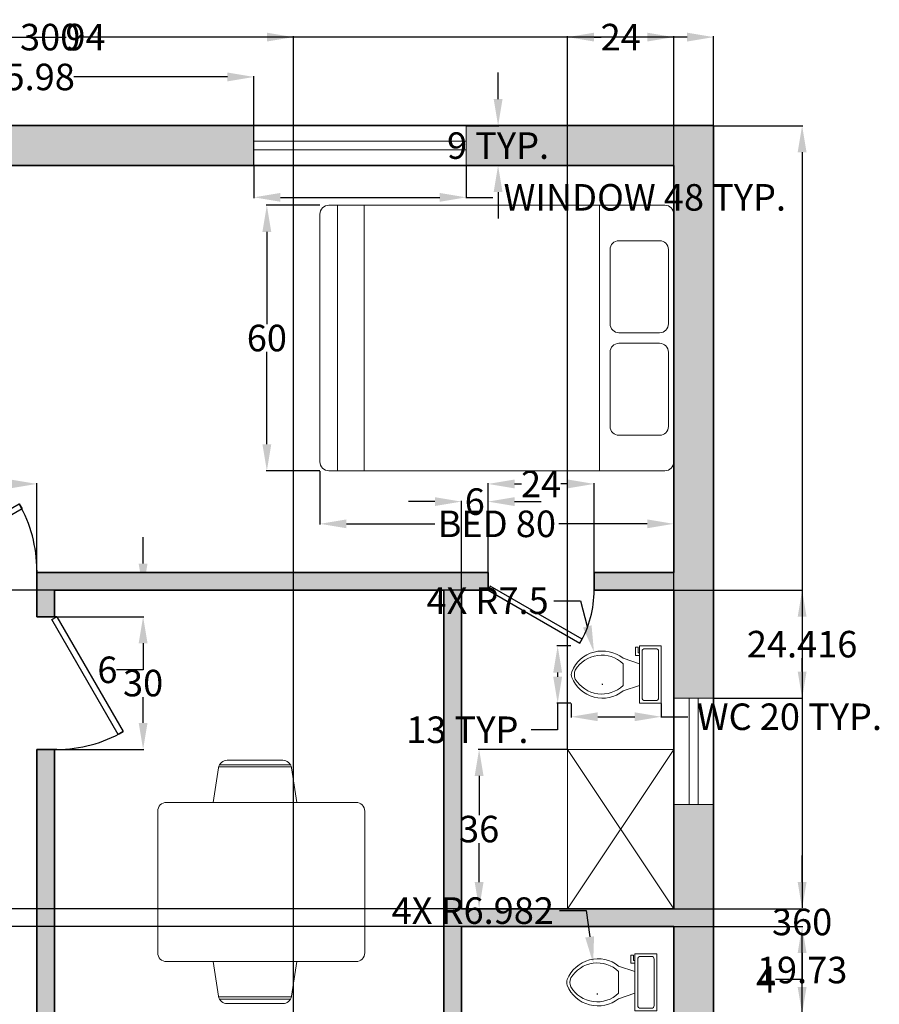
# Model space of a CAD drawing. Units: inches. Extents: x -26 to 363, y -399 to 37.
# Tile 4 of 4: x 168 to 363, y -185 to 37. Entities that reach past the tile are written whole.
import ezdxf

# ---------------------------------------------------------------- set-up
doc = ezdxf.new("R2010")
doc.units = ezdxf.units.IN
doc.header["$MEASUREMENT"] = 0
for name, color, linetype, lineweight in [('A-ANNO-DIMS', 2, 'Continuous', 18), ('A-DOOR', 3, 'Continuous', 25), ('A-FLOR-FIXT', 9, 'Continuous', 18), ('A-FURN', 8, 'Continuous', 18), ('A-GLAZ', 4, 'Continuous', 18), ('A-WALL', 7, 'Continuous', 35), ('A-WALL-PATT', 251, 'Continuous', 13)]:
    doc.layers.add(name, color=color, linetype=linetype, lineweight=lineweight)
doc.styles.get("Standard").update_dxf_attribs({"font": 'arial.ttf'})
doc.dimstyles.get("Standard").update_dxf_attribs({"dimtxt": 6, "dimasz": 6, "dimexe": 0.18, "dimexo": 0.0625, "dimgap": 0.09, "dimtad": 0, "dimtih": 1, "dimtoh": 1, "dimdec": 0, "dimzin": 0, "dimdsep": 46, "dimlunit": 4, "dimtxsty": 'Standard', "dimcen": 0.09, "dimadec": 0, "dimazin": 0, "dimtfac": 1, "dimtdec": 0, "dimtofl": 0, "dimtmove": 0, "dimatfit": 3, "dimfxl": 1, "dimtolj": 1, "dimtzin": 0, "dimarcsym": 0})

# ---------------------------------------------------------------- blocks, each defined once
blk = doc.blocks.new('*U3')
for p, q in [((0, 0), (0, 6)), ((40, 0), (40, 6))]:
    blk.add_line(p, q)
blk.add_lwpolyline([(0, 0), (34.64, -20), (35.52, -18.48), (0.87, 1.52)], close=True)
blk.add_arc((0, 0), 40, 330, 0)
blk = doc.blocks.new('*U2')
for p, q in [((0, 0), (0, -6)), ((40, 0), (40, -6))]:
    blk.add_line(p, q)
blk.add_lwpolyline([(0, 0), (34.64, 20), (35.52, 18.48), (0.87, -1.52)], close=True)
blk.add_arc((0, 0), 40, 0, 30)
blk = doc.blocks.new('Toilet - top')
for p, q in [((9.5, -6), (9.5, -2)), ((-10, -8.5), (-8, -8.5)), ((-10, -9.5), (-10, -8.5)), ((-7, -9.5), (-10, -9.5)), ((-8, -8.5), (-8, -8)), ((-7, -8), (-7, -9.5)), ((-4, -8), (-6, -14)), ((4, -8), (6, -14)), ((4, -14), (-4, -14))]:
    blk.add_line(p, q)
blk.add_lwpolyline([(10.5, -8), (10.5, 0), (-10.5, 0), (-10.5, -8)], close=True)
for points in [[(-9.5, -2), (-9.5, -6)], [(8.5, -1), (-8.5, -1)], [(-8.5, -7), (8.5, -7)]]:
    blk.add_lwpolyline(points)
for centre, radius, start, end in [((-8.62, -1.88), 0.884, 81.8699, 188.1301), ((8.62, -1.88), 0.884, 351.8699, 98.1301), ((-8.62, -6.12), 0.884, 171.8699, 278.1301), ((8.62, -6.12), 0.884, 261.8699, 8.1301), ((3.52, -21.58), 12.17, 141.4691, 247.9714), ((4.2, -21.82), 11.33, 136.3677, 238.9468), ((-3.52, -21.58), 12.17, 292.0284, 38.5307), ((-4.2, -21.82), 11.33, 301.053, 43.6321), ((0, -27.88), 4, 245.7318, 294.2682), ((0, -29), 4, 254.8605, 285.1395)]:
    blk.add_arc(centre, radius, start, end)
blk = doc.blocks.new('Bed - Queen')
for p, q in [((2, 0), (57.99999, 0)), ((0, -78.00003), (0, -2)), ((9.99999, -1.2), (26.79998, -1.2)), ((33.19999, -1.2), (49.99999, -1.2)), ((59.99999, -2), (59.99999, -78.00003)), ((7.99999, -12.4), (7.99999, -3.2)), ((28.79998, -3.2), (28.79998, -12.4)), ((31.19999, -12.4), (31.19999, -3.2)), ((51.99999, -3.2), (51.99999, -12.4)), ((9.99999, -14.4), (26.79998, -14.4)), ((33.19999, -14.4), (49.99999, -14.4)), ((59.99999, -16.8), (0, -16.8)), ((59.99999, -70.00003), (0, -70.00003)), ((59.99999, -76.00003), (0, -76.00003)), ((57.99999, -80.00003), (2, -80.00003))]:
    blk.add_line(p, q)
for centre, start, end in [((2, -2), 90, 180), ((57.99999, -2), 0, 90), ((9.99999, -3.2), 90, 180), ((26.79998, -3.2), 0, 90), ((33.19999, -3.2), 90, 180), ((49.99999, -3.2), 0, 90), ((9.99999, -12.4), 180, 270), ((26.79998, -12.4), 270, 0), ((33.19999, -12.4), 180, 270), ((49.99999, -12.4), 270, 0), ((2, -78.00003), 180, 270), ((57.99999, -78.00003), 270, 0)]:
    blk.add_arc(centre, 2, start, end)
blk = doc.blocks.new('WIN-48IN')
for p, q in [((0, 0), (0, 9)), ((48, 9), (48, 0)), ((48, 5.5), (0, 5.5)), ((48, 3.5), (0, 3.5))]:
    blk.add_line(p, q)
blk = doc.blocks.new('WIN-24IN')
for p, q in [((0, 24), (9, 24)), ((3.5, 24), (3.5, 0)), ((5.5, 24), (5.5, 0)), ((9, 0), (0, 0))]:
    blk.add_line(p, q)
blk = doc.blocks.new('*D17')
at = {"layer": 'A-ANNO-DIMS', "color": 0, "lineweight": -2, "transparency": 16777216}
for p, q in [((221.4, 4.38), (221.4, -2.94)), ((269.4, 4.38), (269.4, -2.94)), ((227.4, -2.76), (263.4, -2.76)), ((269.4, -2.76), (275.4, -2.76))]:
    blk.add_line(p, q, dxfattribs=at)
at = {"layer": 'A-ANNO-DIMS', "color": 0, "transparency": 16777216}
for points in [[(227.4, -1.76), (227.4, -3.76), (221.4, -2.76)], [(263.4, -1.76), (263.4, -3.76), (269.4, -2.76)]]:
    blk.add_solid(points, dxfattribs=at)
at = {"layer": 'Defpoints', "color": 0, "transparency": 16777216}
for p in [(221.4, 4.44), (269.4, 4.44), (269.4, -2.76)]:
    blk.add_point(p, dxfattribs=at)
at = {"layer": 'A-ANNO-DIMS', "color": 0, "transparency": 16777216, "insert": (309.77, -2.76), "char_height": 6, "attachment_point": 5}
blk.add_mtext('\\A1;WINDOW 48 TYP.', dxfattribs=at)
blk = doc.blocks.new('*D18')
at = {"layer": 'A-ANNO-DIMS', "color": 0, "lineweight": -2, "transparency": 16777216}
for p, q in [((276.6, 19.44), (276.6, 25.44)), ((269.47, 13.44), (276.78, 13.44)), ((269.47, 4.44), (276.78, 4.44)), ((276.6, -1.56), (276.6, -7.56))]:
    blk.add_line(p, q, dxfattribs=at)
at = {"layer": 'A-ANNO-DIMS', "color": 0, "transparency": 16777216}
for points in [[(275.6, 19.44), (277.6, 19.44), (276.6, 13.44)], [(275.6, -1.56), (277.6, -1.56), (276.6, 4.44)]]:
    blk.add_solid(points, dxfattribs=at)
at = {"layer": 'Defpoints', "color": 0, "transparency": 16777216}
for p in [(269.4, 13.44), (276.6, 13.44), (269.4, 4.44)]:
    blk.add_point(p, dxfattribs=at)
at = {"layer": 'A-ANNO-DIMS', "color": 0, "transparency": 16777216, "insert": (276.6, 8.94), "char_height": 6, "attachment_point": 5}
blk.add_mtext('\\A1;9 TYP.', dxfattribs=at)
blk = doc.blocks.new('*D21')
at = {"layer": 'A-ANNO-DIMS', "color": 0, "lineweight": -2, "transparency": 16777216}
for p, q in [((236.32, -64.62), (236.32, -76.74)), ((316.32, -64.62), (316.32, -76.74)), ((242.32, -76.56), (262.3, -76.56)), ((310.32, -76.56), (290.35, -76.56))]:
    blk.add_line(p, q, dxfattribs=at)
at = {"layer": 'A-ANNO-DIMS', "color": 0, "transparency": 16777216}
for points in [[(242.32, -75.56), (242.32, -77.56), (236.32, -76.56)], [(310.32, -75.56), (310.32, -77.56), (316.32, -76.56)]]:
    blk.add_solid(points, dxfattribs=at)
at = {"layer": 'Defpoints', "color": 0, "transparency": 16777216}
for p in [(236.32, -64.56), (316.32, -64.56), (316.32, -76.56)]:
    blk.add_point(p, dxfattribs=at)
at = {"layer": 'A-ANNO-DIMS', "color": 0, "transparency": 16777216, "insert": (276.32, -76.56), "char_height": 6, "attachment_point": 5}
blk.add_mtext('\\A1;BED 80', dxfattribs=at)
blk = doc.blocks.new('*D22')
at = {"layer": 'A-ANNO-DIMS', "color": 0, "lineweight": -2, "transparency": 16777216}
for p, q in [((236.26, -4.56), (224.14, -4.56)), ((224.32, -10.56), (224.32, -31.4)), ((224.32, -58.56), (224.32, -37.71)), ((236.26, -64.56), (224.14, -64.56))]:
    blk.add_line(p, q, dxfattribs=at)
at = {"layer": 'A-ANNO-DIMS', "color": 0, "transparency": 16777216}
for points in [[(223.32, -10.56), (225.32, -10.56), (224.32, -4.56)], [(223.32, -58.56), (225.32, -58.56), (224.32, -64.56)]]:
    blk.add_solid(points, dxfattribs=at)
at = {"layer": 'Defpoints', "color": 0, "transparency": 16777216}
for p in [(236.32, -4.56), (224.32, -64.56), (236.32, -64.56)]:
    blk.add_point(p, dxfattribs=at)
at = {"layer": 'A-ANNO-DIMS', "color": 0, "transparency": 16777216, "insert": (224.32, -34.56), "char_height": 6, "attachment_point": 5}
blk.add_mtext('\\A1;60', dxfattribs=at)
blk = doc.blocks.new('*D27')
at = {"layer": 'A-ANNO-DIMS', "color": 0, "lineweight": -2, "transparency": 16777216}
for p, q in [((293.13, -117.17), (293.13, -120.35)), ((313.49, -117.17), (313.49, -120.35)), ((299.13, -120.17), (307.49, -120.17)), ((313.49, -120.17), (319.49, -120.17))]:
    blk.add_line(p, q, dxfattribs=at)
at = {"layer": 'A-ANNO-DIMS', "color": 0, "transparency": 16777216}
for points in [[(299.13, -119.17), (299.13, -121.17), (293.13, -120.17)], [(307.49, -119.17), (307.49, -121.17), (313.49, -120.17)]]:
    blk.add_solid(points, dxfattribs=at)
at = {"layer": 'Defpoints', "color": 0, "transparency": 16777216}
for p in [(293.13, -117.11), (313.49, -117.11), (313.49, -120.17)]:
    blk.add_point(p, dxfattribs=at)
at = {"layer": 'A-ANNO-DIMS', "color": 0, "transparency": 16777216, "insert": (342.46, -120.17), "char_height": 6, "attachment_point": 5}
blk.add_mtext('\\A1;WC 20 TYP.', dxfattribs=at)
blk = doc.blocks.new('*D28')
at = {"layer": 'A-ANNO-DIMS', "color": 0, "lineweight": -2, "transparency": 16777216}
for p, q in [((293.07, -104.17), (289.89, -104.17)), ((290.07, -110.17), (290.07, -111.11)), ((293.07, -117.11), (289.89, -117.11)), ((290.07, -117.11), (290.07, -123.11)), ((290.07, -123.11), (284.07, -123.11))]:
    blk.add_line(p, q, dxfattribs=at)
at = {"layer": 'A-ANNO-DIMS', "color": 0, "transparency": 16777216}
for points in [[(289.07, -110.17), (291.07, -110.17), (290.07, -104.17)], [(289.07, -111.11), (291.07, -111.11), (290.07, -117.11)]]:
    blk.add_solid(points, dxfattribs=at)
at = {"layer": 'Defpoints', "color": 0, "transparency": 16777216}
for p in [(293.13, -104.17), (290.07, -117.11), (293.13, -117.11)]:
    blk.add_point(p, dxfattribs=at)
at = {"layer": 'A-ANNO-DIMS', "color": 0, "transparency": 16777216, "insert": (269.66, -123.11), "char_height": 6, "attachment_point": 5}
blk.add_mtext('\\A1;13 TYP.', dxfattribs=at)
blk = doc.blocks.new('*D39')
at = {"layer": 'A-ANNO-DIMS', "color": 0, "lineweight": -2, "transparency": 16777216}
for p, q in [((25.32, 13.51), (25.32, 33.64)), ((31.32, 33.46), (168.62, 33.46)), ((319.32, 33.46), (182.03, 33.46)), ((325.32, 13.51), (325.32, 33.64))]:
    blk.add_line(p, q, dxfattribs=at)
at = {"layer": 'A-ANNO-DIMS', "color": 0, "transparency": 16777216}
for points in [[(31.32, 34.46), (31.32, 32.46), (25.32, 33.46)], [(319.32, 34.46), (319.32, 32.46), (325.32, 33.46)]]:
    blk.add_solid(points, dxfattribs=at)
at = {"layer": 'Defpoints', "color": 0, "transparency": 16777216}
for p in [(325.32, 33.46), (25.32, 13.44), (325.32, 13.44)]:
    blk.add_point(p, dxfattribs=at)
at = {"layer": 'A-ANNO-DIMS', "color": 0, "transparency": 16777216, "insert": (175.32, 33.46), "char_height": 6, "attachment_point": 5}
blk.add_mtext('\\A1;300', dxfattribs=at)
blk = doc.blocks.new('*D41')
at = {"layer": 'A-ANNO-DIMS', "color": 0, "lineweight": -2, "transparency": 16777216}
for p, q in [((325.39, 13.44), (345.52, 13.44)), ((345.34, 7.44), (345.34, -163.4)), ((345.34, -340.56), (345.34, -169.71)), ((325.39, -346.56), (345.52, -346.56))]:
    blk.add_line(p, q, dxfattribs=at)
at = {"layer": 'A-ANNO-DIMS', "color": 0, "transparency": 16777216}
for points in [[(344.34, 7.44), (346.34, 7.44), (345.34, 13.44)], [(344.34, -340.56), (346.34, -340.56), (345.34, -346.56)]]:
    blk.add_solid(points, dxfattribs=at)
at = {"layer": 'Defpoints', "color": 0, "transparency": 16777216}
for p in [(325.32, 13.44), (345.34, 13.44), (325.32, -346.56)]:
    blk.add_point(p, dxfattribs=at)
at = {"layer": 'A-ANNO-DIMS', "color": 0, "transparency": 16777216, "insert": (345.34, -166.56), "char_height": 6, "attachment_point": 5}
blk.add_mtext('\\A1;360', dxfattribs=at)
blk = doc.blocks.new('*D48')
at = {"layer": 'A-ANNO-DIMS', "color": 0, "lineweight": -2, "transparency": 16777216}
for p, q in [((176.26, -91.56), (156.13, -91.56)), ((156.31, -97.56), (156.31, -141.4)), ((156.31, -191.56), (156.31, -147.71)), ((176.26, -197.56), (156.13, -197.56))]:
    blk.add_line(p, q, dxfattribs=at)
at = {"layer": 'A-ANNO-DIMS', "color": 0, "transparency": 16777216}
for points in [[(155.31, -97.56), (157.31, -97.56), (156.31, -91.56)], [(155.31, -191.56), (157.31, -191.56), (156.31, -197.56)]]:
    blk.add_solid(points, dxfattribs=at)
at = {"layer": 'Defpoints', "color": 0, "transparency": 16777216}
for p in [(156.31, -91.56), (176.32, -91.56), (176.32, -197.56)]:
    blk.add_point(p, dxfattribs=at)
at = {"layer": 'A-ANNO-DIMS', "color": 0, "transparency": 16777216, "insert": (156.31, -144.56), "char_height": 6, "attachment_point": 5}
blk.add_mtext('\\A1;106', dxfattribs=at)
blk = doc.blocks.new('*D50')
at = {"layer": 'A-ANNO-DIMS', "color": 0, "lineweight": -2, "transparency": 16777216}
for p, q in [((268.26, -91.56), (5.13, -91.56)), ((5.31, -97.56), (5.31, -124.45)), ((5.31, -157.56), (5.31, -130.66)), ((268.26, -163.56), (5.13, -163.56))]:
    blk.add_line(p, q, dxfattribs=at)
at = {"layer": 'A-ANNO-DIMS', "color": 0, "transparency": 16777216}
for points in [[(4.31, -97.56), (6.31, -97.56), (5.31, -91.56)], [(4.31, -157.56), (6.31, -157.56), (5.31, -163.56)]]:
    blk.add_solid(points, dxfattribs=at)
at = {"layer": 'Defpoints', "color": 0, "transparency": 16777216}
for p in [(268.32, -91.56), (5.31, -163.56), (268.32, -163.56)]:
    blk.add_point(p, dxfattribs=at)
at = {"layer": 'A-ANNO-DIMS', "color": 0, "transparency": 16777216, "insert": (5.31, -127.56), "char_height": 6, "attachment_point": 5}
blk.add_mtext('\\A1;72', dxfattribs=at)
blk = doc.blocks.new('*D51')
at = {"layer": 'A-ANNO-DIMS', "color": 0, "lineweight": -2, "transparency": 16777216}
for p, q in [((268.26, -167.56), (5.13, -167.56)), ((5.31, -173.56), (5.31, -196.4)), ((5.31, -225.56), (5.31, -202.71)), ((268.26, -231.56), (5.13, -231.56))]:
    blk.add_line(p, q, dxfattribs=at)
at = {"layer": 'A-ANNO-DIMS', "color": 0, "transparency": 16777216}
for points in [[(4.31, -173.56), (6.31, -173.56), (5.31, -167.56)], [(4.31, -225.56), (6.31, -225.56), (5.31, -231.56)]]:
    blk.add_solid(points, dxfattribs=at)
at = {"layer": 'Defpoints', "color": 0, "transparency": 16777216}
for p in [(268.32, -167.56), (5.31, -231.56), (268.32, -231.56)]:
    blk.add_point(p, dxfattribs=at)
at = {"layer": 'A-ANNO-DIMS', "color": 0, "transparency": 16777216, "insert": (5.31, -199.56), "char_height": 6, "attachment_point": 5}
blk.add_mtext('\\A1;64', dxfattribs=at)
blk = doc.blocks.new('*D54')
at = {"layer": 'A-ANNO-DIMS', "color": 0, "lineweight": -2, "transparency": 16777216}
for p, q in [((115.43, 4.51), (115.43, 24.64)), ((221.4, 4.51), (221.4, 24.64)), ((121.43, 24.46), (156.15, 24.46)), ((215.4, 24.46), (180.68, 24.46))]:
    blk.add_line(p, q, dxfattribs=at)
at = {"layer": 'A-ANNO-DIMS', "color": 0, "transparency": 16777216}
for points in [[(121.43, 25.46), (121.43, 23.46), (115.43, 24.46)], [(215.4, 25.46), (215.4, 23.46), (221.4, 24.46)]]:
    blk.add_solid(points, dxfattribs=at)
at = {"layer": 'Defpoints', "color": 0, "transparency": 16777216}
for p in [(221.4, 24.46), (115.43, 4.44), (221.4, 4.44)]:
    blk.add_point(p, dxfattribs=at)
at = {"layer": 'A-ANNO-DIMS', "color": 0, "transparency": 16777216, "insert": (168.42, 24.46), "char_height": 6, "attachment_point": 5}
blk.add_mtext('\\A1;105.98', dxfattribs=at)
blk = doc.blocks.new('*D57')
at = {"layer": 'A-ANNO-DIMS', "color": 0, "lineweight": -2, "transparency": 16777216}
for p, q in [((316.39, -91.56), (345.52, -91.56)), ((345.34, -97.56), (345.34, -100.61)), ((345.34, -109.97), (345.34, -106.92)), ((325.39, -115.97), (345.52, -115.97))]:
    blk.add_line(p, q, dxfattribs=at)
at = {"layer": 'A-ANNO-DIMS', "color": 0, "transparency": 16777216}
for points in [[(344.34, -97.56), (346.34, -97.56), (345.34, -91.56)], [(344.34, -109.97), (346.34, -109.97), (345.34, -115.97)]]:
    blk.add_solid(points, dxfattribs=at)
at = {"layer": 'Defpoints', "color": 0, "transparency": 16777216}
for p in [(316.32, -91.56), (345.34, -91.56), (325.32, -115.97)]:
    blk.add_point(p, dxfattribs=at)
at = {"layer": 'A-ANNO-DIMS', "color": 0, "transparency": 16777216, "insert": (345.34, -103.76), "char_height": 6, "attachment_point": 5}
blk.add_mtext('\\A1;24.416', dxfattribs=at)
blk = doc.blocks.new('*D58')
at = {"layer": 'A-ANNO-DIMS', "color": 0, "lineweight": -2, "transparency": 16777216}
for p, q in [((316.39, -167.56), (345.52, -167.56)), ((345.34, -173.56), (345.34, -174.26)), ((345.34, -181.28), (345.34, -180.58)), ((325.39, -187.28), (345.52, -187.28))]:
    blk.add_line(p, q, dxfattribs=at)
at = {"layer": 'A-ANNO-DIMS', "color": 0, "transparency": 16777216}
for points in [[(344.34, -173.56), (346.34, -173.56), (345.34, -167.56)], [(344.34, -181.28), (346.34, -181.28), (345.34, -187.28)]]:
    blk.add_solid(points, dxfattribs=at)
at = {"layer": 'Defpoints', "color": 0, "transparency": 16777216}
for p in [(316.32, -167.56), (345.34, -167.56), (325.32, -187.28)]:
    blk.add_point(p, dxfattribs=at)
at = {"layer": 'A-ANNO-DIMS', "color": 0, "transparency": 16777216, "insert": (345.34, -177.42), "char_height": 6, "attachment_point": 5}
blk.add_mtext('\\A1;19.73', dxfattribs=at)
blk = doc.blocks.new('*D61')
at = {"layer": 'A-ANNO-DIMS', "color": 0, "lineweight": -2, "transparency": 16777216}
for p, q in [((142.32, -87.49), (142.32, -67.36)), ((148.32, -67.54), (152.95, -67.54)), ((166.32, -67.54), (161.7, -67.54)), ((172.32, -87.49), (172.32, -67.36))]:
    blk.add_line(p, q, dxfattribs=at)
at = {"layer": 'A-ANNO-DIMS', "color": 0, "transparency": 16777216}
for points in [[(148.32, -66.54), (148.32, -68.54), (142.32, -67.54)], [(166.32, -66.54), (166.32, -68.54), (172.32, -67.54)]]:
    blk.add_solid(points, dxfattribs=at)
at = {"layer": 'Defpoints', "color": 0, "transparency": 16777216}
for p in [(172.32, -67.54), (142.32, -87.56), (172.32, -87.56)]:
    blk.add_point(p, dxfattribs=at)
at = {"layer": 'A-ANNO-DIMS', "color": 0, "transparency": 16777216, "insert": (157.32, -67.54), "char_height": 6, "attachment_point": 5}
blk.add_mtext('\\A1;30', dxfattribs=at)
blk = doc.blocks.new('*D62')
at = {"layer": 'A-ANNO-DIMS', "color": 0, "lineweight": -2, "transparency": 16777216}
for p, q in [((274.32, -87.49), (274.32, -67.36)), ((280.32, -67.54), (281.9, -67.54)), ((292.32, -67.54), (290.75, -67.54)), ((298.32, -87.49), (298.32, -67.36))]:
    blk.add_line(p, q, dxfattribs=at)
at = {"layer": 'A-ANNO-DIMS', "color": 0, "transparency": 16777216}
for points in [[(280.32, -66.54), (280.32, -68.54), (274.32, -67.54)], [(292.32, -66.54), (292.32, -68.54), (298.32, -67.54)]]:
    blk.add_solid(points, dxfattribs=at)
at = {"layer": 'Defpoints', "color": 0, "transparency": 16777216}
for p in [(298.32, -67.54), (274.32, -87.56), (298.32, -87.56)]:
    blk.add_point(p, dxfattribs=at)
at = {"layer": 'A-ANNO-DIMS', "color": 0, "transparency": 16777216, "insert": (286.32, -67.54), "char_height": 6, "attachment_point": 5}
blk.add_mtext('\\A1;24', dxfattribs=at)
blk = doc.blocks.new('*D63')
at = {"layer": 'A-ANNO-DIMS', "color": 0, "lineweight": -2, "transparency": 16777216}
for p, q in [((176.39, -97.56), (196.52, -97.56)), ((196.34, -103.56), (196.34, -109.4)), ((196.34, -121.56), (196.34, -115.71)), ((176.39, -127.56), (196.52, -127.56))]:
    blk.add_line(p, q, dxfattribs=at)
at = {"layer": 'A-ANNO-DIMS', "color": 0, "transparency": 16777216}
for points in [[(195.34, -103.56), (197.34, -103.56), (196.34, -97.56)], [(195.34, -121.56), (197.34, -121.56), (196.34, -127.56)]]:
    blk.add_solid(points, dxfattribs=at)
at = {"layer": 'Defpoints', "color": 0, "transparency": 16777216}
for p in [(176.32, -97.56), (176.32, -127.56), (196.34, -127.56)]:
    blk.add_point(p, dxfattribs=at)
at = {"layer": 'A-ANNO-DIMS', "color": 0, "transparency": 16777216, "insert": (196.34, -112.56), "char_height": 6, "attachment_point": 5}
blk.add_mtext('\\A1;30', dxfattribs=at)
blk = doc.blocks.new('*D66')
at = {"layer": 'A-ANNO-DIMS', "color": 0, "lineweight": -2, "transparency": 16777216}
for p, q in [((292.32, -127.49), (292.32, 33.64)), ((298.32, 33.46), (299.9, 33.46)), ((310.32, 33.46), (308.75, 33.46)), ((316.32, -127.49), (316.32, 33.64))]:
    blk.add_line(p, q, dxfattribs=at)
at = {"layer": 'A-ANNO-DIMS', "color": 0, "transparency": 16777216}
for points in [[(298.32, 34.46), (298.32, 32.46), (292.32, 33.46)], [(310.32, 34.46), (310.32, 32.46), (316.32, 33.46)]]:
    blk.add_solid(points, dxfattribs=at)
at = {"layer": 'Defpoints', "color": 0, "transparency": 16777216}
for p in [(316.32, 33.46), (292.32, -127.56), (316.32, -127.56)]:
    blk.add_point(p, dxfattribs=at)
at = {"layer": 'A-ANNO-DIMS', "color": 0, "transparency": 16777216, "insert": (304.32, 33.46), "char_height": 6, "attachment_point": 5}
blk.add_mtext('\\A1;24', dxfattribs=at)
blk = doc.blocks.new('*D67')
at = {"layer": 'A-ANNO-DIMS', "color": 0, "lineweight": -2, "transparency": 16777216}
for p, q in [((292.26, -127.56), (272.13, -127.56)), ((272.31, -133.56), (272.31, -142.4)), ((272.31, -157.56), (272.31, -148.71)), ((292.26, -163.56), (272.13, -163.56))]:
    blk.add_line(p, q, dxfattribs=at)
at = {"layer": 'A-ANNO-DIMS', "color": 0, "transparency": 16777216}
for points in [[(271.31, -133.56), (273.31, -133.56), (272.31, -127.56)], [(271.31, -157.56), (273.31, -157.56), (272.31, -163.56)]]:
    blk.add_solid(points, dxfattribs=at)
at = {"layer": 'Defpoints', "color": 0, "transparency": 16777216}
for p in [(272.31, -127.56), (292.32, -127.56), (292.32, -163.56)]:
    blk.add_point(p, dxfattribs=at)
at = {"layer": 'A-ANNO-DIMS', "color": 0, "transparency": 16777216, "insert": (272.31, -145.56), "char_height": 6, "attachment_point": 5}
blk.add_mtext('\\A1;36', dxfattribs=at)
blk = doc.blocks.new('*D69')
at = {"layer": 'A-ANNO-DIMS', "color": 0, "lineweight": -2, "transparency": 16777216}
for p, q in [((345.34, -157.56), (345.34, -151.56)), ((316.39, -163.56), (345.52, -163.56)), ((316.39, -167.56), (345.52, -167.56)), ((345.34, -173.56), (345.34, -179.56)), ((345.34, -179.56), (339.34, -179.56))]:
    blk.add_line(p, q, dxfattribs=at)
at = {"layer": 'A-ANNO-DIMS', "color": 0, "transparency": 16777216}
for points in [[(344.34, -157.56), (346.34, -157.56), (345.34, -163.56)], [(344.34, -173.56), (346.34, -173.56), (345.34, -167.56)]]:
    blk.add_solid(points, dxfattribs=at)
at = {"layer": 'Defpoints', "color": 0, "transparency": 16777216}
for p in [(316.32, -163.56), (316.32, -167.56), (345.34, -167.56)]:
    blk.add_point(p, dxfattribs=at)
at = {"layer": 'A-ANNO-DIMS', "color": 0, "transparency": 16777216, "insert": (337.17, -179.56), "char_height": 6, "attachment_point": 5}
blk.add_mtext('\\A1;4', dxfattribs=at)
blk = doc.blocks.new('*D76')
at = {"layer": 'A-ANNO-DIMS', "color": 0, "lineweight": -2, "transparency": 16777216}
for p, q in [((136.32, -337.49), (136.32, 33.64)), ((142.32, 33.46), (178.95, 33.46)), ((224.32, 33.46), (187.7, 33.46)), ((230.32, -337.49), (230.32, 33.64))]:
    blk.add_line(p, q, dxfattribs=at)
at = {"layer": 'A-ANNO-DIMS', "color": 0, "transparency": 16777216}
for points in [[(142.32, 34.46), (142.32, 32.46), (136.32, 33.46)], [(224.32, 34.46), (224.32, 32.46), (230.32, 33.46)]]:
    blk.add_solid(points, dxfattribs=at)
at = {"layer": 'Defpoints', "color": 0, "transparency": 16777216}
for p in [(230.32, 33.46), (136.32, -337.56), (230.32, -337.56)]:
    blk.add_point(p, dxfattribs=at)
at = {"layer": 'A-ANNO-DIMS', "color": 0, "transparency": 16777216, "insert": (183.32, 33.46), "char_height": 6, "attachment_point": 5}
blk.add_mtext('\\A1;94', dxfattribs=at)
blk = doc.blocks.new('*D77')
at = {"layer": 'A-ANNO-DIMS', "color": 0, "lineweight": -2, "transparency": 16777216}
for p, q in [((262.322775, -71.538613), (256.322775, -71.538613)), ((268.322775, -91.492613), (268.322775, -71.358613)), ((274.322775, -91.492613), (274.322775, -71.358613)), ((280.322775, -71.538613), (286.322775, -71.538613))]:
    blk.add_line(p, q, dxfattribs=at)
at = {"layer": 'A-ANNO-DIMS', "color": 0, "transparency": 16777216}
for points in [[(262.322775, -70.538613), (262.322775, -72.538613), (268.322775, -71.538613)], [(280.322775, -70.538613), (280.322775, -72.538613), (274.322775, -71.538613)]]:
    blk.add_solid(points, dxfattribs=at)
at = {"layer": 'Defpoints', "color": 0, "transparency": 16777216}
for p in [(274.322775, -71.538613), (268.322775, -91.555113), (274.322775, -91.555113)]:
    blk.add_point(p, dxfattribs=at)
at = {"layer": 'A-ANNO-DIMS', "color": 0, "transparency": 16777216, "insert": (271.322775, -71.538613), "char_height": 6, "attachment_point": 5}
blk.add_mtext('\\A1;6', dxfattribs=at)
blk = doc.blocks.new('*D82')
at = {"layer": 'A-ANNO-DIMS', "color": 0, "lineweight": -2, "transparency": 16777216}
for p, q in [((196.34, -85.56), (196.34, -79.56)), ((176.39, -91.56), (196.52, -91.56)), ((176.39, -97.56), (196.52, -97.56)), ((196.34, -103.56), (196.34, -109.56)), ((196.34, -109.56), (190.34, -109.56))]:
    blk.add_line(p, q, dxfattribs=at)
at = {"layer": 'A-ANNO-DIMS', "color": 0, "transparency": 16777216}
for points in [[(195.34, -85.56), (197.34, -85.56), (196.34, -91.56)], [(195.34, -103.56), (197.34, -103.56), (196.34, -97.56)]]:
    blk.add_solid(points, dxfattribs=at)
at = {"layer": 'Defpoints', "color": 0, "transparency": 16777216}
for p in [(176.32, -91.56), (176.32, -97.56), (196.34, -97.56)]:
    blk.add_point(p, dxfattribs=at)
at = {"layer": 'A-ANNO-DIMS', "color": 0, "transparency": 16777216, "insert": (188.27, -109.56), "char_height": 6, "attachment_point": 5}
blk.add_mtext('\\A1;6', dxfattribs=at)
blk = doc.blocks.new('*D83')
at = {"layer": 'A-ANNO-DIMS', "color": 0, "lineweight": -2, "transparency": 16777216}
for p, q in [((289.24, -93.95), (295.24, -93.95)), ((295.24, -93.95), (296.76, -99.75)), ((300.1, -112.81), (300.28, -112.81)), ((300.19, -112.9), (300.19, -112.72))]:
    blk.add_line(p, q, dxfattribs=at)
at = {"layer": 'A-ANNO-DIMS', "color": 0, "transparency": 16777216}
blk.add_solid([(297.73, -99.5), (295.8, -100.01), (298.29, -105.56)], dxfattribs=at)
at = {"layer": 'Defpoints', "color": 0, "transparency": 16777216}
for p in [(298.29, -105.56), (300.19, -112.81)]:
    blk.add_point(p, dxfattribs=at)
at = {"layer": 'A-ANNO-DIMS', "color": 0, "transparency": 16777216, "insert": (274.23, -93.95), "char_height": 6, "attachment_point": 5}
blk.add_mtext('\\A1;4X R7.5', dxfattribs=at)
blk = doc.blocks.new('*D84')
at = {"layer": 'A-ANNO-DIMS', "color": 0, "lineweight": -2, "transparency": 16777216}
for p, q in [((290.51, -163.99), (296.51, -163.99)), ((296.51, -163.99), (297.31, -169.94)), ((298.95, -182.8), (299.13, -182.8)), ((299.04, -182.89), (299.04, -182.71))]:
    blk.add_line(p, q, dxfattribs=at)
at = {"layer": 'A-ANNO-DIMS', "color": 0, "transparency": 16777216}
blk.add_solid([(298.3, -169.8), (296.31, -170.07), (298.1, -175.88)], dxfattribs=at)
at = {"layer": 'Defpoints', "color": 0, "transparency": 16777216}
for p in [(298.1, -175.88), (299.04, -182.8)]:
    blk.add_point(p, dxfattribs=at)
at = {"layer": 'A-ANNO-DIMS', "color": 0, "transparency": 16777216, "insert": (270.88, -163.99), "char_height": 6, "attachment_point": 5}
blk.add_mtext('\\A1;4X R6.982', dxfattribs=at)

msp = doc.modelspace()

# ---------------------------------------------------------------- hatches: boundary and pattern name
at = {"layer": 'A-WALL-PATT'}
h = msp.add_hatch(color=256, dxfattribs=at)
h.dxf.hatch_style = 1
h.paths.add_polyline_path([(221.4046, 13.4449), (115.429, 13.4449), (115.429, 4.4449), (132.3228, 4.4449), (132.3228, -87.5551), (126.3228, -87.5551), (126.3228, -91.5551), (142.3228, -91.5551), (142.3228, -87.5551), (136.3228, -87.5551), (136.3228, 4.4449), (221.4046, 4.4449)])
h = msp.add_hatch(color=256, dxfattribs=at)
h.dxf.hatch_style = 1
h.paths.add_polyline_path([(325.3228, 13.4449), (269.4046, 13.4449), (269.4046, 4.4449), (316.3228, 4.4449), (316.3228, -87.5551), (298.3228, -87.5551), (298.3228, -91.5551), (316.3228, -91.5551), (316.3228, -115.9712), (325.3228, -115.9712)])
h = msp.add_hatch(color=256, dxfattribs=at)
h.dxf.hatch_style = 1
h.paths.add_polyline_path([(325.3228, -139.9712), (316.3228, -139.9712), (316.3228, -163.5551), (292.3228, -163.5551), (268.3228, -163.5551), (268.3228, -91.5551), (274.3228, -91.5551), (274.3228, -87.5551), (172.3228, -87.5551), (172.3228, -91.5551), (172.3228, -97.5551), (176.3228, -97.5551), (176.3228, -91.5551), (264.3228, -91.5551), (264.3228, -197.5551), (258.3228, -197.5551), (176.3228, -197.5551), (176.3228, -127.5551), (172.3228, -127.5551), (172.3228, -197.5551), (172.3228, -201.5551), (258.3228, -201.5551), (264.3228, -201.5551), (268.3228, -201.5551), (268.3228, -167.5551), (316.3228, -167.5551), (316.3228, -187.2842), (325.3228, -187.2842)])

# ---------------------------------------------------------------- linework, layer by layer
at = {"layer": 'A-FLOR-FIXT'}
for p, q in [((292.3228, -127.5551), (316.3228, -163.5551)), ((316.3228, -127.5551), (292.3228, -163.5551))]:
    msp.add_line(p, q, dxfattribs=at)
msp.add_lwpolyline([(316.3228, -127.5551), (292.3228, -127.5551), (292.3228, -163.5551), (316.3228, -163.5551)], close=True, dxfattribs=at)
at = {"layer": 'A-FURN'}
for p, q in [((229.6555, -131.0173), (213.6149, -131.0173)), ((215.3469, -130.0173), (227.9234, -130.0173)), ((229.7936, -131.0173), (229.7914, -131.0173)), ((229.7915, -131.0176), (229.7914, -131.0173)), ((213.3709, -131.7085), (212.1505, -139.5197)), ((213.4048, -131.5173), (229.8744, -131.5173)), ((231.12, -139.5197), (229.8994, -131.7085)), ((244.4676, -139.5173), (201.6352, -139.5173)), ((244.4676, -139.5173), (236.4597, -139.5173)), ((199.6352, -141.5173), (199.6352, -173.5173)), ((246.4676, -173.5173), (246.4676, -141.5173)), ((201.6352, -175.5173), (236.4597, -175.5173)), ((213.3709, -183.326), (212.1505, -175.5149)), ((231.12, -175.5149), (229.8994, -183.326)), ((236.4597, -175.5173), (244.4676, -175.5173)), ((213.4048, -183.5173), (229.8599, -183.5173)), ((229.6555, -184.0173), (213.6149, -184.0173)), ((215.3469, -185.0173), (227.9234, -185.0173))]:
    msp.add_line(p, q, dxfattribs=at)
for centre, start, end in [((215.3469, -132.0173), 90, 171.119789), ((227.9234, -132.0173), 8.880965, 90), ((201.6352, -141.5173), 90, 180), ((244.4676, -141.5173), 0, 90), ((201.6352, -173.5173), 180, 270), ((244.4676, -173.5173), 270, 0), ((215.3469, -183.0173), 188.880201, 270), ((227.9234, -183.0173), 270, 351.119057)]:
    msp.add_arc(centre, 2, start, end, dxfattribs=at)
at = {"layer": 'A-WALL'}
for p, q in [((136.3228, 4.4449), (316.3228, 4.4449)), ((316.3228, 4.4449), (316.3228, -87.5551)), ((172.3228, -87.5551), (172.3228, -91.5551)), ((172.3228, -87.5551), (274.3228, -87.5551)), ((274.3228, -91.5551), (274.3228, -87.5551)), ((298.3228, -91.5551), (298.3228, -87.5551)), ((298.3228, -87.5551), (316.3228, -87.5551)), ((172.3228, -97.5551), (172.3228, -91.5551)), ((176.3228, -91.5551), (264.3228, -91.5551)), ((176.3228, -97.5551), (176.3228, -91.5551)), ((264.3228, -91.5551), (264.3228, -197.5551)), ((268.3228, -91.5551), (268.3228, -163.5551)), ((268.3228, -91.5551), (274.3228, -91.5551)), ((298.3228, -91.5551), (316.3228, -91.5551)), ((316.3228, -91.5551), (316.3228, -163.5551)), ((176.3228, -97.5551), (172.3228, -97.5551)), ((172.3228, -197.5551), (172.3228, -127.5551)), ((176.3228, -127.5551), (172.3228, -127.5551)), ((176.3228, -197.5551), (176.3228, -127.5551)), ((268.3228, -163.5551), (316.3228, -163.5551)), ((268.3228, -167.5551), (316.3228, -167.5551)), ((268.3228, -167.5551), (268.3228, -201.5551)), ((316.3228, -167.5551), (316.3228, -231.5551))]:
    msp.add_line(p, q, dxfattribs=at)
msp.add_lwpolyline([(25.3228, -315.3126), (25.3228, 13.4449), (325.3228, 13.4449), (325.3228, -346.5551), (220.3228, -346.5551)], dxfattribs=at)

# ---------------------------------------------------------------- block references
at = {"layer": 'A-DOOR'}
for name, p, xscale, yscale, zscale in [('*U2', (142.3228, -87.0551), 0.75, 0.75, 0.75), ('*U3', (274.3228, -91.5551), 0.6, 0.6, 0.6)]:
    msp.add_blockref(name, p, dxfattribs=dict(at, xscale=xscale, yscale=yscale, zscale=zscale))
at = {"layer": 'A-DOOR', "xscale": 0.75, "yscale": 0.75, "zscale": 0.75, "rotation": 270}
msp.add_blockref('*U2', (176.8228, -97.5551), dxfattribs=at)
at = {"layer": 'A-FLOR-FIXT', "xscale": 0.6163129826161287, "yscale": 0.6163129826161287, "zscale": 0.6163129826161287, "rotation": 270}
for p in [(313.4944, -110.6406), (312.4819, -180.2133)]:
    msp.add_blockref('Toilet - top', p, dxfattribs=at)
at = {"layer": 'A-FURN', "rotation": 270}
msp.add_blockref('Bed - Queen', (316.3228, -4.5561), dxfattribs=at)
at = {"layer": 'A-GLAZ'}
msp.add_blockref('WIN-48IN', (221.4046, 4.445), dxfattribs=at)
at = {"layer": 'A-GLAZ', "rotation": 180}
msp.add_blockref('WIN-24IN', (325.3225, -115.9714), dxfattribs=at)

# ---------------------------------------------------------------- dimensions: what is measured, and where the dimension line sits
at = {"layer": 'A-ANNO-DIMS'}
for base, p1, p2, picture, middle in [((325.3228, 33.4614), (25.3228, 13.4449), (325.3228, 13.4449), '*D39', (175.3228, 33.4614)), ((230.3228, 33.4614), (136.3228, -337.5551), (230.3228, -337.5551), '*D76', (183.3228, 33.4614)), ((316.3228, 33.4614), (292.3228, -127.5551), (316.3228, -127.5551), '*D66', (304.3228, 33.4614)), ((172.3228, -67.5386), (142.3228, -87.5551), (172.3228, -87.5551), '*D61', (157.3228, -67.5386)), ((298.3228, -67.5386), (274.3228, -87.5551), (298.3228, -87.5551), '*D62', (286.3228, -67.5386)), ((274.3228, -71.5386), (268.3228, -91.5551), (274.3228, -91.5551), '*D77', (271.3228, -71.5386))]:
    dim = msp.add_linear_dim(base=base, p1=p1, p2=p2, dimstyle='Standard', override={"dimdec": 0, "dimlfac": 1, "dimrnd": 0, "dimzin": 0, "dimdsep": 46, "dimlunit": 2}, dxfattribs=at)
    dim.commit()
    dim.dimension.update_dxf_attribs({"geometry": picture, "text_midpoint": middle})
for base, p1, p2, angle, override, picture, middle in [((221.4046, 24.4614), (115.429, 4.4449), (221.4046, 4.4449), 0, {"dimdec": 2, "dimlfac": 1, "dimrnd": 0, "dimzin": 0, "dimdsep": 46, "dimlunit": 2}, '*D54', (168.4168, 24.4614)), ((345.3393, 13.4449), (325.3228, -346.5551), (325.3228, 13.4449), 90, {"dimdec": 0, "dimlfac": 1, "dimrnd": 0, "dimzin": 0, "dimdsep": 46, "dimlunit": 2}, '*D41', (345.3393, -166.5551)), ((224.3227, -64.5561), (236.3227, -4.5561), (236.3227, -64.5561), 270, {"dimdec": 0, "dimlfac": 1, "dimrnd": 0, "dimzin": 0, "dimdsep": 46, "dimlunit": 2}, '*D22', (224.3227, -34.5561)), ((196.3393, -97.5551), (176.3228, -91.5551), (176.3228, -97.5551), 270, {"dimdec": 0, "dimlfac": 1, "dimrnd": 0, "dimzin": 0, "dimdsep": 46, "dimlunit": 2}, '*D82', (188.2684, -109.5551)), ((5.3063, -163.5551), (268.3228, -91.5551), (268.3228, -163.5551), 90, {"dimdec": 0, "dimlfac": 1, "dimrnd": 0, "dimzin": 0, "dimdsep": 46, "dimlunit": 2}, '*D50', (5.3063, -127.5551)), ((156.3063, -91.5551), (176.3228, -197.5551), (176.3228, -91.5551), 90, {"dimdec": 0, "dimlfac": 1, "dimrnd": 0, "dimzin": 0, "dimdsep": 46, "dimlunit": 2}, '*D48', (156.3063, -144.5551)), ((345.3393, -91.5551), (325.3228, -115.9712), (316.3228, -91.5551), 90, {"dimdec": 3, "dimlfac": 1, "dimrnd": 0, "dimzin": 0, "dimdsep": 46, "dimlunit": 2}, '*D57', (345.3393, -103.7632)), ((196.3393, -127.5551), (176.3228, -97.5551), (176.3228, -127.5551), 270, {"dimdec": 0, "dimlfac": 1, "dimrnd": 0, "dimzin": 0, "dimdsep": 46, "dimlunit": 2}, '*D63', (196.3393, -112.5551)), ((272.3063, -127.5551), (292.3228, -163.5551), (292.3228, -127.5551), 90, {"dimdec": 0, "dimlfac": 1, "dimrnd": 0, "dimzin": 0, "dimdsep": 46, "dimlunit": 2}, '*D67', (272.3063, -145.5551)), ((345.3393, -167.5551), (316.3228, -163.5551), (316.3228, -167.5551), 90, {"dimdec": 0, "dimlfac": 1, "dimrnd": 0, "dimzin": 0, "dimdsep": 46, "dimlunit": 2}, '*D69', (337.1742, -179.5551)), ((5.3063, -231.5551), (268.3228, -167.5551), (268.3228, -231.5551), 90, {"dimdec": 0, "dimlfac": 1, "dimrnd": 0, "dimzin": 0, "dimdsep": 46, "dimlunit": 2}, '*D51', (5.3063, -199.5551)), ((345.3393, -167.5551), (325.3228, -187.2842), (316.3228, -167.5551), 90, {"dimdec": 2, "dimlfac": 1, "dimrnd": 0, "dimzin": 0, "dimdsep": 46, "dimlunit": 2}, '*D58', (345.3393, -177.4197))]:
    dim = msp.add_linear_dim(base=base, p1=p1, p2=p2, angle=angle, dimstyle='Standard', override=override, dxfattribs=at)
    dim.commit()
    dim.dimension.update_dxf_attribs({"geometry": picture, "text_midpoint": middle})
for base, p1, p2, angle, picture, middle in [((276.6046, 13.4449), (269.4046, 4.4449), (269.4046, 13.4449), 90, '*D18', (276.6046, 8.9449)), ((290.0726, -117.1119), (293.1276, -104.1694), (293.1276, -117.1119), 270, '*D28', (269.662, -123.1119))]:
    dim = msp.add_linear_dim(base=base, p1=p1, p2=p2, angle=angle, text='<> TYP.', dimstyle='Standard', override={"dimdec": 0, "dimlfac": 1, "dimrnd": 0, "dimzin": 0, "dimdsep": 46, "dimlunit": 2}, dxfattribs=at)
    dim.commit()
    dim.dimension.update_dxf_attribs({"geometry": picture, "text_midpoint": middle})
for base, p1, p2, text, picture, middle in [((269.4046, -2.7551), (221.4046, 4.4449), (269.4046, 4.4449), 'WINDOW <> TYP.', '*D17', (309.7736, -2.7551)), ((316.3228, -76.5561), (236.3227, -64.5561), (316.3228, -64.5561), 'BED <>', '*D21', (276.3228, -76.5561)), ((313.4944, -120.167), (293.1276, -117.1119), (313.4944, -117.1119), 'WC <> TYP.', '*D27', (342.4569, -120.167))]:
    dim = msp.add_linear_dim(base=base, p1=p1, p2=p2, text=text, dimstyle='Standard', override={"dimdec": 0, "dimlfac": 1, "dimrnd": 0, "dimzin": 0, "dimdsep": 46, "dimlunit": 2}, dxfattribs=at)
    dim.commit()
    dim.dimension.update_dxf_attribs({"geometry": picture, "text_midpoint": middle})
for center, mpoint, override, picture, middle in [((300.1941, -112.8098), (298.288, -105.5561), {"dimdec": 1, "dimlfac": 1, "dimrnd": 0, "dimzin": 0, "dimdsep": 46, "dimlunit": 2}, '*D83', (274.2261, -93.9501)), ((299.0356, -182.8018), (298.105, -175.8817), {"dimdec": 3, "dimlfac": 1, "dimrnd": 0, "dimzin": 0, "dimdsep": 46, "dimlunit": 2}, '*D84', (270.8849, -163.9888))]:
    dim = msp.add_radius_dim(center=center, mpoint=mpoint, text='4X <>', dimstyle='Standard', override=override, dxfattribs=at)
    dim.commit()
    dim.dimension.update_dxf_attribs({"geometry": picture, "text_midpoint": middle})

doc.saveas('drawing.dxf')
